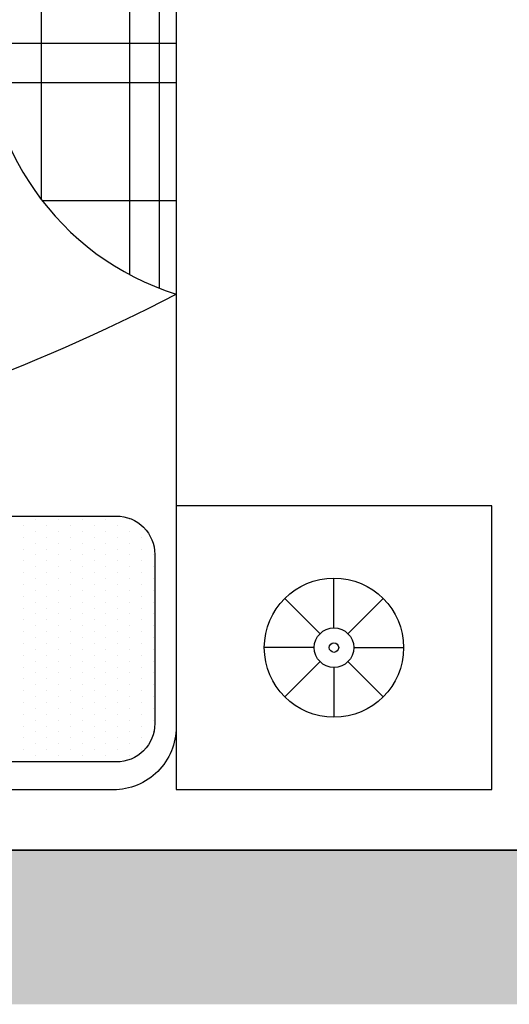
# Model space of a CAD drawing. Units: millimetres. Extents: x 2817 to 5038, y 1110 to 3565.
# Tile 6 of 21: x 2917 to 2946, y 1265 to 1323. Entities that reach past the tile are written whole.
import ezdxf

# ---------------------------------------------------------------- set-up
doc = ezdxf.new("R2010")
doc.units = ezdxf.units.MM
doc.layers.add('A-WALL', color=7, linetype='Continuous', lineweight=35)
doc.layers.add('FURNITURE', color=219, linetype='Continuous', lineweight=18)
doc.layers.add('A-WALL-PATT', color=51, linetype='Continuous', lineweight=13, true_color=0xf7f281)
doc.layers.add('BLOCK', color=6, linetype='Continuous')

# ---------------------------------------------------------------- blocks, each defined once
blk = doc.blocks.new('*X7')
at = {"color": 0}
for p, q in [((276.598, 451.25), (280.51, 451.25)), ((275.455, 450.625), (280.51, 450.625)), ((274.411, 450), (280.51, 450)), ((265.51, 448.125), (267.634, 448.125)), ((271.723, 448.125), (280.51, 448.125)), ((265.51, 446.25), (268.465, 446.25)), ((269.519, 446.25), (280.51, 446.25)), ((265.51, 445.625), (268.531, 445.625)), ((268.866, 445.625), (280.51, 445.625)), ((265.51, 445), (280.51, 445)), ((265.51, 443.125), (280.51, 443.125)), ((265.51, 441.25), (280.51, 441.25)), ((265.51, 440.625), (280.51, 440.625)), ((265.634, 440), (280.386, 440))]:
    blk.add_line(p, q, dxfattribs=at)
blk = doc.blocks.new('*X8')
at = {"color": 0}
for p, q in [((280.312, 439.886), (280.312, 452.896)), ((278.906, 439.482), (278.906, 452.338)), ((277.5, 439.482), (277.5, 451.702)), ((277.031, 439.482), (277.031, 451.471)), ((276.562, 439.482), (276.562, 451.231)), ((275.156, 439.482), (275.156, 450.451)), ((273.75, 439.482), (273.75, 449.576)), ((265.781, 439.797), (265.781, 449.511)), ((266.25, 439.517), (266.25, 449.296)), ((273.281, 439.482), (273.281, 449.261)), ((272.812, 439.482), (272.812, 448.934)), ((267.656, 439.482), (267.656, 448.095)), ((271.406, 439.482), (271.406, 447.876)), ((270, 439.482), (270, 446.689)), ((269.531, 439.482), (269.531, 446.262)), ((269.062, 439.482), (269.062, 445.817))]:
    blk.add_line(p, q, dxfattribs=at)
blk = doc.blocks.new('*X9')
at = {"color": 0}
for p, q in [((266.25, 456.9375), (266.25, 456.9375)), ((266.4375, 457.03125), (266.4375, 457.03125)), ((266.625, 456.9375), (266.625, 456.9375)), ((266.8125, 457.03125), (266.8125, 457.03125)), ((267, 456.9375), (267, 456.9375)), ((267.1875, 457.03125), (267.1875, 457.03125)), ((267.375, 456.9375), (267.375, 456.9375)), ((267.5625, 457.03125), (267.5625, 457.03125)), ((267.75, 456.9375), (267.75, 456.9375)), ((267.9375, 457.03125), (267.9375, 457.03125)), ((266.0625, 456.84375), (266.0625, 456.84375)), ((266.25, 456.75), (266.25, 456.75)), ((266.4375, 456.84375), (266.4375, 456.84375)), ((266.625, 456.75), (266.625, 456.75)), ((266.8125, 456.84375), (266.8125, 456.84375)), ((267, 456.75), (267, 456.75)), ((267.1875, 456.84375), (267.1875, 456.84375)), ((267.375, 456.75), (267.375, 456.75)), ((267.5625, 456.84375), (267.5625, 456.84375)), ((267.75, 456.75), (267.75, 456.75)), ((267.9375, 456.84375), (267.9375, 456.84375)), ((266.0625, 456.65625), (266.0625, 456.65625)), ((266.4375, 456.65625), (266.4375, 456.65625)), ((266.8125, 456.65625), (266.8125, 456.65625)), ((267.1875, 456.65625), (267.1875, 456.65625)), ((267.5625, 456.65625), (267.5625, 456.65625)), ((267.9375, 456.65625), (267.9375, 456.65625)), ((265.875, 456.5625), (265.875, 456.5625)), ((266.0625, 456.46875), (266.0625, 456.46875)), ((266.25, 456.5625), (266.25, 456.5625)), ((266.4375, 456.46875), (266.4375, 456.46875)), ((266.625, 456.5625), (266.625, 456.5625)), ((266.8125, 456.46875), (266.8125, 456.46875)), ((267, 456.5625), (267, 456.5625)), ((267.1875, 456.46875), (267.1875, 456.46875)), ((267.375, 456.5625), (267.375, 456.5625)), ((267.5625, 456.46875), (267.5625, 456.46875)), ((267.75, 456.5625), (267.75, 456.5625)), ((267.9375, 456.46875), (267.9375, 456.46875)), ((265.875, 456.375), (265.875, 456.375)), ((266.0625, 456.28125), (266.0625, 456.28125)), ((266.25, 456.375), (266.25, 456.375)), ((266.4375, 456.28125), (266.4375, 456.28125)), ((266.625, 456.375), (266.625, 456.375)), ((266.8125, 456.28125), (266.8125, 456.28125)), ((267, 456.375), (267, 456.375)), ((267.1875, 456.28125), (267.1875, 456.28125)), ((267.375, 456.375), (267.375, 456.375)), ((267.5625, 456.28125), (267.5625, 456.28125)), ((267.75, 456.375), (267.75, 456.375)), ((267.9375, 456.28125), (267.9375, 456.28125)), ((265.875, 456.1875), (265.875, 456.1875)), ((266.25, 456.1875), (266.25, 456.1875)), ((266.625, 456.1875), (266.625, 456.1875)), ((267, 456.1875), (267, 456.1875)), ((267.375, 456.1875), (267.375, 456.1875)), ((267.75, 456.1875), (267.75, 456.1875)), ((265.875, 456), (265.875, 456)), ((266.0625, 456.09375), (266.0625, 456.09375)), ((266.25, 456), (266.25, 456)), ((266.4375, 456.09375), (266.4375, 456.09375)), ((266.625, 456), (266.625, 456)), ((266.8125, 456.09375), (266.8125, 456.09375)), ((267, 456), (267, 456)), ((267.1875, 456.09375), (267.1875, 456.09375)), ((267.375, 456), (267.375, 456)), ((267.5625, 456.09375), (267.5625, 456.09375)), ((267.75, 456), (267.75, 456)), ((267.9375, 456.09375), (267.9375, 456.09375)), ((265.875, 455.8125), (265.875, 455.8125)), ((266.0625, 455.90625), (266.0625, 455.90625)), ((266.25, 455.8125), (266.25, 455.8125)), ((266.4375, 455.90625), (266.4375, 455.90625)), ((266.625, 455.8125), (266.625, 455.8125)), ((266.8125, 455.90625), (266.8125, 455.90625)), ((267, 455.8125), (267, 455.8125)), ((267.1875, 455.90625), (267.1875, 455.90625)), ((267.375, 455.8125), (267.375, 455.8125)), ((267.5625, 455.90625), (267.5625, 455.90625)), ((267.75, 455.8125), (267.75, 455.8125)), ((267.9375, 455.90625), (267.9375, 455.90625)), ((266.0625, 455.71875), (266.0625, 455.71875)), ((266.4375, 455.71875), (266.4375, 455.71875)), ((266.8125, 455.71875), (266.8125, 455.71875)), ((267.1875, 455.71875), (267.1875, 455.71875)), ((267.5625, 455.71875), (267.5625, 455.71875)), ((267.9375, 455.71875), (267.9375, 455.71875)), ((265.875, 455.625), (265.875, 455.625)), ((266.0625, 455.53125), (266.0625, 455.53125)), ((266.25, 455.625), (266.25, 455.625)), ((266.4375, 455.53125), (266.4375, 455.53125)), ((266.625, 455.625), (266.625, 455.625)), ((266.8125, 455.53125), (266.8125, 455.53125)), ((267, 455.625), (267, 455.625)), ((267.1875, 455.53125), (267.1875, 455.53125)), ((267.375, 455.625), (267.375, 455.625)), ((267.5625, 455.53125), (267.5625, 455.53125)), ((267.75, 455.625), (267.75, 455.625)), ((267.9375, 455.53125), (267.9375, 455.53125)), ((265.875, 455.4375), (265.875, 455.4375)), ((266.0625, 455.34375), (266.0625, 455.34375)), ((266.25, 455.4375), (266.25, 455.4375)), ((266.4375, 455.34375), (266.4375, 455.34375)), ((266.625, 455.4375), (266.625, 455.4375)), ((266.8125, 455.34375), (266.8125, 455.34375)), ((267, 455.4375), (267, 455.4375)), ((267.1875, 455.34375), (267.1875, 455.34375)), ((267.375, 455.4375), (267.375, 455.4375)), ((267.5625, 455.34375), (267.5625, 455.34375)), ((267.75, 455.4375), (267.75, 455.4375)), ((267.9375, 455.34375), (267.9375, 455.34375)), ((265.875, 455.25), (265.875, 455.25)), ((266.25, 455.25), (266.25, 455.25)), ((266.625, 455.25), (266.625, 455.25)), ((267, 455.25), (267, 455.25)), ((267.375, 455.25), (267.375, 455.25)), ((267.75, 455.25), (267.75, 455.25)), ((265.875, 455.0625), (265.875, 455.0625)), ((266.0625, 455.15625), (266.0625, 455.15625)), ((266.25, 455.0625), (266.25, 455.0625)), ((266.4375, 455.15625), (266.4375, 455.15625)), ((266.625, 455.0625), (266.625, 455.0625)), ((266.8125, 455.15625), (266.8125, 455.15625)), ((267, 455.0625), (267, 455.0625)), ((267.1875, 455.15625), (267.1875, 455.15625)), ((267.375, 455.0625), (267.375, 455.0625)), ((267.5625, 455.15625), (267.5625, 455.15625)), ((267.75, 455.0625), (267.75, 455.0625)), ((267.9375, 455.15625), (267.9375, 455.15625)), ((265.875, 454.875), (265.875, 454.875)), ((266.0625, 454.96875), (266.0625, 454.96875)), ((266.25, 454.875), (266.25, 454.875)), ((266.4375, 454.96875), (266.4375, 454.96875)), ((266.625, 454.875), (266.625, 454.875)), ((266.8125, 454.96875), (266.8125, 454.96875)), ((267, 454.875), (267, 454.875)), ((267.1875, 454.96875), (267.1875, 454.96875)), ((267.375, 454.875), (267.375, 454.875)), ((267.5625, 454.96875), (267.5625, 454.96875)), ((267.75, 454.875), (267.75, 454.875)), ((267.9375, 454.96875), (267.9375, 454.96875)), ((266.0625, 454.78125), (266.0625, 454.78125)), ((266.4375, 454.78125), (266.4375, 454.78125)), ((266.8125, 454.78125), (266.8125, 454.78125)), ((267.1875, 454.78125), (267.1875, 454.78125)), ((267.5625, 454.78125), (267.5625, 454.78125)), ((267.9375, 454.78125), (267.9375, 454.78125)), ((265.875, 454.6875), (265.875, 454.6875)), ((266.0625, 454.59375), (266.0625, 454.59375)), ((266.25, 454.6875), (266.25, 454.6875)), ((266.4375, 454.59375), (266.4375, 454.59375)), ((266.625, 454.6875), (266.625, 454.6875)), ((266.8125, 454.59375), (266.8125, 454.59375)), ((267, 454.6875), (267, 454.6875)), ((267.1875, 454.59375), (267.1875, 454.59375)), ((267.375, 454.6875), (267.375, 454.6875)), ((267.5625, 454.59375), (267.5625, 454.59375)), ((267.75, 454.6875), (267.75, 454.6875)), ((267.9375, 454.59375), (267.9375, 454.59375)), ((265.875, 454.5), (265.875, 454.5)), ((266.0625, 454.40625), (266.0625, 454.40625)), ((266.25, 454.5), (266.25, 454.5)), ((266.4375, 454.40625), (266.4375, 454.40625)), ((266.625, 454.5), (266.625, 454.5)), ((266.8125, 454.40625), (266.8125, 454.40625)), ((267, 454.5), (267, 454.5)), ((267.1875, 454.40625), (267.1875, 454.40625)), ((267.375, 454.5), (267.375, 454.5)), ((267.5625, 454.40625), (267.5625, 454.40625)), ((267.75, 454.5), (267.75, 454.5)), ((267.9375, 454.40625), (267.9375, 454.40625)), ((265.875, 454.3125), (265.875, 454.3125)), ((266.25, 454.3125), (266.25, 454.3125)), ((266.625, 454.3125), (266.625, 454.3125)), ((267, 454.3125), (267, 454.3125)), ((267.375, 454.3125), (267.375, 454.3125)), ((267.75, 454.3125), (267.75, 454.3125)), ((265.875, 454.125), (265.875, 454.125)), ((266.0625, 454.21875), (266.0625, 454.21875)), ((266.25, 454.125), (266.25, 454.125)), ((266.4375, 454.21875), (266.4375, 454.21875)), ((266.625, 454.125), (266.625, 454.125)), ((266.8125, 454.21875), (266.8125, 454.21875)), ((267, 454.125), (267, 454.125)), ((267.1875, 454.21875), (267.1875, 454.21875)), ((267.375, 454.125), (267.375, 454.125)), ((267.5625, 454.21875), (267.5625, 454.21875)), ((267.75, 454.125), (267.75, 454.125)), ((267.9375, 454.21875), (267.9375, 454.21875)), ((265.875, 453.9375), (265.875, 453.9375)), ((266.0625, 454.03125), (266.0625, 454.03125)), ((266.25, 453.9375), (266.25, 453.9375)), ((266.4375, 454.03125), (266.4375, 454.03125)), ((266.625, 453.9375), (266.625, 453.9375)), ((266.8125, 454.03125), (266.8125, 454.03125)), ((267, 453.9375), (267, 453.9375)), ((267.1875, 454.03125), (267.1875, 454.03125)), ((267.375, 453.9375), (267.375, 453.9375)), ((267.5625, 454.03125), (267.5625, 454.03125)), ((267.75, 453.9375), (267.75, 453.9375)), ((267.9375, 454.03125), (267.9375, 454.03125)), ((266.0625, 453.84375), (266.0625, 453.84375)), ((266.4375, 453.84375), (266.4375, 453.84375)), ((266.8125, 453.84375), (266.8125, 453.84375)), ((267.1875, 453.84375), (267.1875, 453.84375)), ((267.5625, 453.84375), (267.5625, 453.84375)), ((267.9375, 453.84375), (267.9375, 453.84375)), ((265.875, 453.75), (265.875, 453.75)), ((266.0625, 453.65625), (266.0625, 453.65625)), ((266.25, 453.75), (266.25, 453.75)), ((266.4375, 453.65625), (266.4375, 453.65625)), ((266.625, 453.75), (266.625, 453.75)), ((266.8125, 453.65625), (266.8125, 453.65625)), ((267, 453.75), (267, 453.75)), ((267.1875, 453.65625), (267.1875, 453.65625)), ((267.375, 453.75), (267.375, 453.75)), ((267.5625, 453.65625), (267.5625, 453.65625)), ((267.75, 453.75), (267.75, 453.75)), ((267.9375, 453.65625), (267.9375, 453.65625)), ((266.0625, 453.46875), (266.0625, 453.46875)), ((266.25, 453.5625), (266.25, 453.5625)), ((266.4375, 453.46875), (266.4375, 453.46875)), ((266.625, 453.5625), (266.625, 453.5625)), ((266.8125, 453.46875), (266.8125, 453.46875)), ((267, 453.5625), (267, 453.5625)), ((267.1875, 453.46875), (267.1875, 453.46875)), ((267.375, 453.5625), (267.375, 453.5625)), ((267.5625, 453.46875), (267.5625, 453.46875)), ((267.75, 453.5625), (267.75, 453.5625)), ((267.9375, 453.46875), (267.9375, 453.46875)), ((266.25, 453.375), (266.25, 453.375)), ((266.625, 453.375), (266.625, 453.375)), ((267, 453.375), (267, 453.375)), ((267.375, 453.375), (267.375, 453.375)), ((267.75, 453.375), (267.75, 453.375)), ((266.0625, 453.28125), (266.0625, 453.28125)), ((266.25, 453.1875), (266.25, 453.1875)), ((266.4375, 453.28125), (266.4375, 453.28125)), ((266.625, 453.1875), (266.625, 453.1875)), ((266.8125, 453.28125), (266.8125, 453.28125)), ((267, 453.1875), (267, 453.1875)), ((267.1875, 453.28125), (267.1875, 453.28125)), ((267.375, 453.1875), (267.375, 453.1875)), ((267.5625, 453.28125), (267.5625, 453.28125)), ((267.75, 453.1875), (267.75, 453.1875)), ((267.9375, 453.28125), (267.9375, 453.28125))]:
    blk.add_line(p, q, dxfattribs=at)
blk = doc.blocks.new('A$C52E67D0D')
at = {"layer": 'BLOCK'}
for p, q in [((250.5, 1605.5), (250.5, 1684.7)), ((228.3, 1596.3), (172.3, 1652.3)), ((272.7, 1596.3), (328.7, 1652.3)), ((219.1, 1574.1), (139.9, 1574.1)), ((281.9, 1574.1), (361.1, 1574.1)), ((228.3, 1551.9), (172.3, 1495.9)), ((272.7, 1551.9), (328.7, 1495.9)), ((250.5, 1542.8), (250.5, 1463.5))]:
    blk.add_line(p, q, dxfattribs=at)
blk.add_lwpolyline([(501, 1348.6), (501, 1799.6), (0, 1799.6), (0, 1348.6)], close=True, dxfattribs=at)
for points in [[(1901, 0), (601, 0, -0.414214), (501, 100), (501, 1700, -0.414214), (601, 1800), (1901, 1800, -0.414214), (2001, 1700), (2001, 100, -0.414214)], [(1171.8, 1365.1), (595.8, 1365.1, -0.414214), (535, 1425.9), (535, 1694.8, -0.414214), (595.8, 1755.7), (1171.8, 1755.7, -0.414214), (1232.6, 1694.8), (1232.6, 1425.9, -0.414214)]]:
    blk.add_lwpolyline(points, format="xyb", close=True, dxfattribs=at)
for radius in [110.6, 31.4, 7.46]:
    blk.add_circle((250.5, 1574.1), radius, dxfattribs=at)
for centre, radius, start, end in [((1888.6, -1664.5), 3015.3, 87.8642, 117.4001), ((371.4, 600.4), 432, 357.3792, 72.5379)]:
    blk.add_arc(centre, radius, start, end, dxfattribs=at)
at = {"layer": 'BLOCK', "xscale": 100, "yscale": 100, "zscale": 100}
for name in ['*X9', '*X8', '*X7']:
    blk.add_blockref(name, (-26050, -43948.2), dxfattribs=at)

msp = doc.modelspace()

# ---------------------------------------------------------------- hatches: boundary and pattern name
at = {"layer": 'A-WALL-PATT'}
h = msp.add_hatch(color=256, dxfattribs=at)
h.dxf.hatch_style = 1
h.paths.add_polyline_path([(3186.7393, 1614.4357), (2841.7393, 1614.4357), (2841.7393, 1568.614), (2850.7393, 1568.7609), (2850.7393, 1605.4357), (2982.7393, 1605.4357), (2991.7393, 1605.4357), (3052.2393, 1605.4357), (3052.2393, 1573.7835), (3061.2393, 1573.7835), (3061.2393, 1605.4357), (3182.2393, 1605.4357), (3182.2393, 1143.4357), (3181.2393, 1143.4357), (3181.2393, 1134.4357), (3186.7393, 1134.4357)])
h.paths.add_polyline_path([(3061.2393, 1143.4357), (3061.2393, 1147.4357), (3052.2393, 1147.4357), (3052.2393, 1143.4357), (2850.7393, 1143.4357), (2850.7393, 1145.2996), (2841.7393, 1145.2996), (2841.7393, 1134.4357), (3061.2393, 1134.4357)], flags=17)
h.paths.add_polyline_path([(2850.7393, 1265.4357), (2946.7393, 1265.4357), (2946.7393, 1270.8357), (2946.7393, 1274.4357), (2850.7393, 1274.4357), (2850.7381, 1274.4357), (2850.7381, 1274.2564), (2841.7393, 1274.2564), (2841.7393, 1193.1527), (2850.7393, 1193.2996)], flags=17)
h.paths.add_polyline_path([(3061.2393, 1299.098), (3052.2393, 1299.098), (3052.2393, 1274.4357), (2991.7393, 1274.4357), (2991.7393, 1340.4357), (2982.7393, 1340.4357), (2982.7393, 1274.4357), (2982.7393, 1265.4357), (3052.2393, 1265.4357), (3052.2393, 1259.143), (3061.2393, 1259.2899)], flags=17)
h.paths.add_polyline_path([(3061.2393, 1383.4357), (3052.2393, 1383.4357), (3052.2393, 1379.4357), (2931.7393, 1379.4357), (2922.7393, 1379.4357), (2850.7393, 1379.4357), (2850.7381, 1379.4357), (2850.7381, 1379.3646), (2841.7393, 1379.3646), (2841.7393, 1322.1095), (2850.7393, 1322.2564), (2850.7393, 1370.4357), (2982.7393, 1370.4357), (2987.2393, 1370.4357), (3017.2393, 1370.4357), (3052.2393, 1370.4357), (3052.2393, 1323.098), (3061.2393, 1323.098)], flags=17)

# ---------------------------------------------------------------- linework, layer by layer
at = {"layer": 'A-WALL'}
msp.add_line((2850.7393, 1274.4357), (2946.7393, 1274.4357), dxfattribs=at)

# ---------------------------------------------------------------- block references
at = {"layer": 'FURNITURE', "xscale": 0.0367705835331598, "yscale": 0.0367705835331598, "zscale": 0.0367705835331598, "rotation": 180}
msp.add_blockref('A$C52E67D0D', (2944.6948, 1344.1495), dxfattribs=at)

doc.saveas('drawing.dxf')
